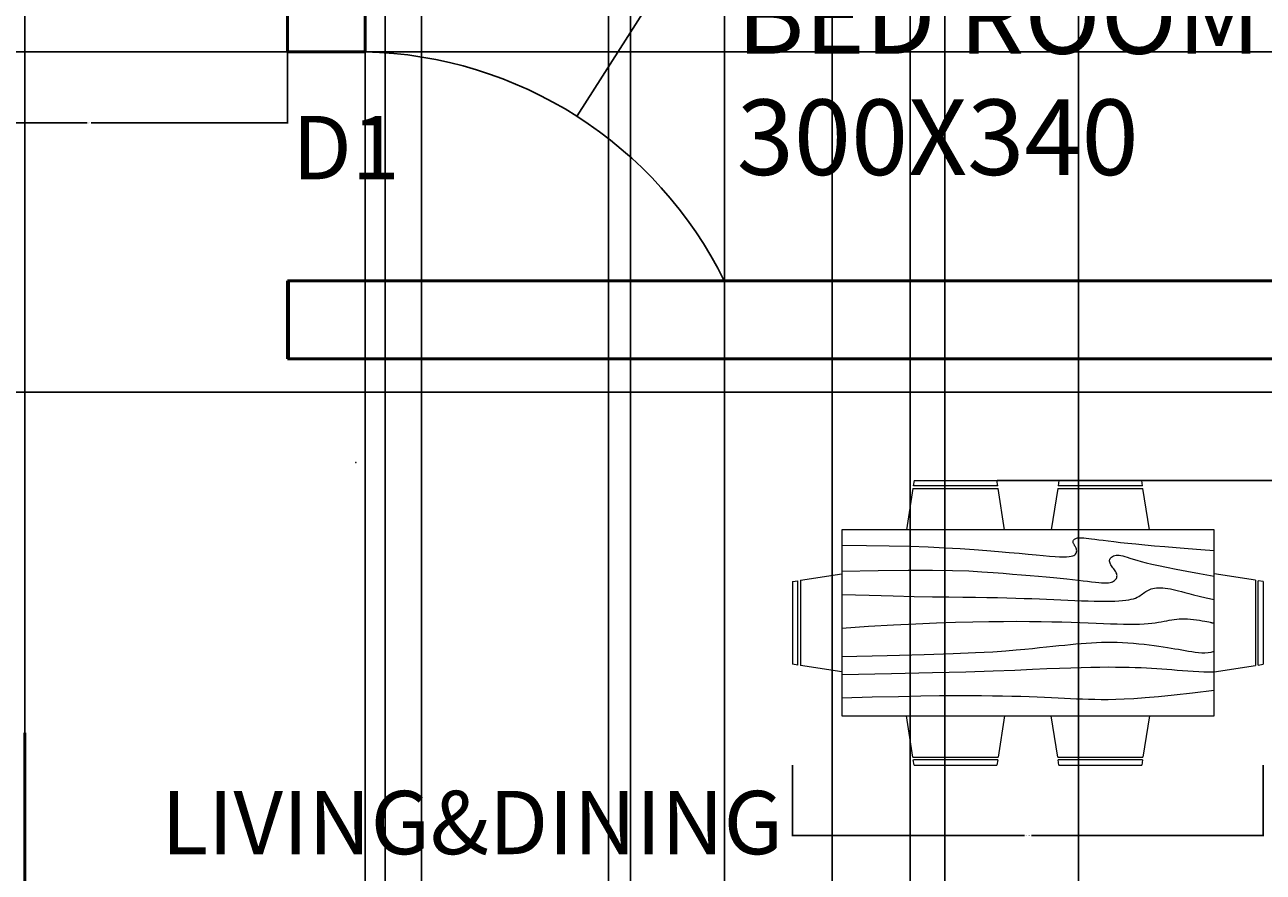
# Model space of a CAD drawing. Units: centimetres. Extents: x 2050 to 3144, y 831 to 2296.
# Tile 4 of 7: x 2553 to 2916, y 1401 to 1650. Entities that reach past the tile are written whole.
import ezdxf

# ---------------------------------------------------------------- set-up
doc = ezdxf.new("R2010")
doc.units = ezdxf.units.CM
for name, color, linetype, lineweight in [('A-ANNO-DIMS', 2, 'Continuous', 18), ('A-ANNO-TEXT', 7, 'Continuous', 18), ('A-AREA-IDEN', 7, 'Continuous', 25), ('A-DOOR', 3, 'Continuous', 25), ('A-FURN', 8, 'Continuous', 18), ('A-WALL', 7, 'Continuous', 50)]:
    doc.layers.add(name, color=color, linetype=linetype, lineweight=lineweight)
doc.styles.get("Standard").update_dxf_attribs({"font": 'arial.ttf'})
doc.dimstyles.get("Standard").update_dxf_attribs({"dimtxt": 0.18, "dimasz": 0.18, "dimexe": 0.18, "dimexo": 0.0625, "dimgap": 0.09, "dimtad": 0, "dimtih": 1, "dimtoh": 1, "dimdec": 4, "dimzin": 0, "dimdsep": 46, "dimtxsty": 'Standard', "dimcen": 0.09, "dimadec": 0, "dimazin": 0, "dimtfac": 1, "dimtdec": 4, "dimtofl": 0, "dimtmove": 0, "dimatfit": 3, "dimfxl": 1, "dimtolj": 1, "dimtzin": 0, "dimarcsym": 0})

# ---------------------------------------------------------------- blocks, each defined once
blk = doc.blocks.new('Dining Set - 36 x 72 in.')
for p, q in [((-22, 27.5), (-22.1562, 26.50042)), ((-5.8416, 26.5), (-22.1534, 26.5)), ((-22, 27.5), (-6, 27.5)), ((-5.8437, 26.49966), (-6, 27.5)), ((6, 27.5), (5.8438, 26.50042)), ((22.1584, 26.5), (5.8466, 26.5)), ((6, 27.5), (22, 27.5)), ((22.1563, 26.49966), (22, 27.5)), ((-22.2343, 26.00059), (-23.4847, 17.99762)), ((-22.2304, 26), (-5.7608, 26)), ((-4.5152, 17.99762), (-5.7655, 25.99926)), ((5.7657, 26.00059), (4.5153, 17.99762)), ((5.7696, 26), (22.2392, 26)), ((23.4848, 17.99762), (22.2345, 25.99926)), ((36, 18), (-36, 18)), ((-36, 18), (-36, -18)), ((36, -18), (36, 18)), ((-45.5, 8), (-44.5004, 8.15617)), ((-45.5, 8), (-45.5, -8)), ((-44.5, -8.15843), (-44.5, 8.15338)), ((-44.0006, 8.23428), (-35.9976, 9.48474)), ((-44, 8.23041), (-44, -8.23915)), ((44.0006, 8.23428), (35.9976, 9.48474)), ((44, 8.23041), (44, -8.23915)), ((44.5, -8.15843), (44.5, 8.15338)), ((45.5, 8), (44.5005, 8.15617)), ((45.5, 8), (45.5, -8)), ((-44.4997, -8.15631), (-45.5, -8)), ((-35.9976, -9.48476), (-43.9993, -8.2345)), ((35.9976, -9.48476), (43.9993, -8.2345)), ((44.4997, -8.15631), (45.5, -8)), ((-36, -18), (36, -18)), ((-22.2343, -26.0006), (-23.4847, -17.99762)), ((-4.5152, -17.99762), (-5.7655, -25.99928)), ((5.7657, -26.0006), (4.5153, -17.99762)), ((23.4848, -17.99762), (22.2345, -25.99928)), ((-22.2304, -26), (-5.7608, -26)), ((5.7696, -26), (22.2392, -26)), ((-22, -27.5), (-22.1562, -26.50044)), ((-5.8416, -26.5), (-22.1534, -26.5)), ((-22, -27.5), (-6, -27.5)), ((-5.8437, -26.49967), (-6, -27.5)), ((6, -27.5), (5.8438, -26.50044)), ((22.1584, -26.5), (5.8466, -26.5)), ((6, -27.5), (22, -27.5)), ((22.1563, -26.49967), (22, -27.5))]:
    blk.add_line(p, q)
for points in [[(-36, 15), (-31.1772, 14.97754), (-26.8079, 14.91406), (-22.8538, 14.81543), (-19.276, 14.6875), (-16.0362, 14.53613), (-13.0957, 14.36718), (-10.4159, 14.18652), (-7.9583, 14), (-5.6904, 13.81315), (-3.6035, 13.63021), (-1.6954, 13.45508), (0.0365, 13.29166), (1.5945, 13.14388), (2.9811, 13.01562), (4.1988, 12.9108), (5.25, 12.83333), (6.1393, 12.78613), (6.8802, 12.76823), (7.4883, 12.77767), (7.9792, 12.8125), (8.3685, 12.87077), (8.6719, 12.95052), (8.9049, 13.0498), (9.0833, 13.16666), (9.2205, 13.29899), (9.3216, 13.44401), (9.3895, 13.59879), (9.4271, 13.76041), (9.4373, 13.92594), (9.4232, 14.09245), (9.3875, 14.257), (9.3333, 14.41666), (9.2638, 14.56917), (9.1836, 14.71484), (9.0975, 14.85465), (9.0104, 14.98958), (8.9272, 15.1206), (8.8529, 15.2487), (8.7922, 15.37483), (8.75, 15.5), (8.7305, 15.62467), (8.7344, 15.74739), (8.7617, 15.86621), (8.8125, 15.97916), (8.8867, 16.08431), (8.9844, 16.17968), (9.1055, 16.26334), (9.25, 16.33333), (9.4189, 16.38802), (9.6172, 16.42708), (9.8506, 16.45052), (10.125, 16.45833), (10.4463, 16.45052), (10.8203, 16.42708), (11.2529, 16.38802), (11.75, 16.33333), (12.3184, 16.26318), (12.9694, 16.17838), (13.7151, 16.07991), (14.5677, 15.96875), (15.5395, 15.84586), (16.6426, 15.71224), (17.8893, 15.56884), (19.2917, 15.41666), (20.859, 15.25667), (22.5879, 15.08984), (24.4721, 14.91715), (26.5052, 14.73958), (28.6809, 14.5581), (30.9929, 14.3737), (33.4347, 14.18733), (36, 14)], [(-36, 10), (-28.9766, 10.14274), (-23.1725, 10.20442), (-18.4241, 10.19775), (-14.5677, 10.13541), (-11.4399, 10.03011), (-8.877, 9.89453), (-6.7154, 9.74137), (-4.7917, 9.58333), (-2.9698, 9.43082), (-1.2246, 9.28515), (0.4415, 9.14534), (2.026, 9.01041), (3.5266, 8.87939), (4.9408, 8.7513), (6.266, 8.62516), (7.5, 8.5), (8.6411, 8.37549), (9.6914, 8.2539), (10.6538, 8.13818), (11.5312, 8.03125), (12.3267, 7.93603), (13.043, 7.85547), (13.6831, 7.79248), (14.25, 7.75), (14.7471, 7.7303), (15.1797, 7.73307), (15.5537, 7.75732), (15.875, 7.80208), (16.1494, 7.86637), (16.3828, 7.94922), (16.5811, 8.04964), (16.75, 8.16666), (16.8944, 8.29915), (17.0143, 8.44531), (17.1089, 8.60319), (17.1771, 8.77083), (17.218, 8.94629), (17.2305, 9.1276), (17.2137, 9.31282), (17.1667, 9.5), (17.0895, 9.6875), (16.987, 9.875), (16.8649, 10.0625), (16.7292, 10.25), (16.5856, 10.4375), (16.4401, 10.625), (16.2985, 10.8125), (16.1667, 11), (16.05, 11.18733), (15.9518, 11.3737), (15.8752, 11.5581), (15.8229, 11.73958), (15.798, 11.91715), (15.8034, 12.08984), (15.842, 12.25667), (15.9167, 12.41666), (16.0295, 12.56836), (16.1784, 12.70833), (16.3605, 12.83268), (16.5729, 12.9375), (16.8127, 13.01888), (17.0768, 13.07291), (17.3625, 13.0957), (17.6667, 13.08333), (17.9894, 13.03312), (18.3418, 12.94726), (18.7382, 12.82918), (19.1927, 12.68229), (19.7195, 12.51001), (20.3327, 12.31575), (21.0465, 12.10294), (21.875, 11.875), (22.8357, 11.63354), (23.959, 11.37304), (25.2786, 11.08618), (26.8282, 10.76562), (28.6414, 10.40405), (30.752, 9.99414), (33.1936, 9.52856), (36, 9)], [(-36, 5.5), (-30.7157, 5.3348), (-26.069, 5.20963), (-21.9946, 5.11767), (-18.4271, 5.05208), (-15.3009, 5.00602), (-12.5508, 4.97265), (-10.1112, 4.94515), (-7.9167, 4.91666), (-5.909, 4.88167), (-4.0586, 4.83984), (-2.3429, 4.79215), (-0.7396, 4.73958), (0.7739, 4.6831), (2.22, 4.6237), (3.6213, 4.56233), (5, 4.5), (6.373, 4.43782), (7.7344, 4.3776), (9.0723, 4.32129), (10.375, 4.27083), (11.6309, 4.22819), (12.8281, 4.19531), (13.9551, 4.17415), (15, 4.16666), (15.954, 4.17448), (16.819, 4.19791), (17.6001, 4.23698), (18.3021, 4.29166), (18.9299, 4.36198), (19.4883, 4.44791), (19.9823, 4.54948), (20.4167, 4.66666), (20.7969, 4.79899), (21.1302, 4.94401), (21.4245, 5.09879), (21.6875, 5.26041), (21.9271, 5.42594), (22.1511, 5.59245), (22.3672, 5.757), (22.5834, 5.91666), (22.8065, 6.06868), (23.0404, 6.21093), (23.2879, 6.34147), (23.5521, 6.45833), (23.8358, 6.55957), (24.142, 6.64323), (24.4735, 6.70735), (24.8334, 6.75), (25.2235, 6.76969), (25.642, 6.76692), (26.0858, 6.74267), (26.5521, 6.69791), (27.0379, 6.63362), (27.5404, 6.55078), (28.0565, 6.45036), (28.5834, 6.33333), (29.1242, 6.19987), (29.7071, 6.04687), (30.3661, 5.87044), (31.1354, 5.66666), (32.0493, 5.43164), (33.142, 5.16146), (34.4475, 4.85221), (36, 4.5)], [(-36, -1), (-30.7915, -0.6591), (-26.0195, -0.38216), (-21.6519, -0.16284), (-17.6563, 0.00521), (-14.0005, 0.12833), (-10.6523, 0.21289), (-7.5796, 0.26522), (-4.75, 0.29166), (-2.134, 0.29793), (0.2878, 0.28711), (2.5317, 0.26163), (4.6146, 0.22396), (6.5529, 0.17651), (8.3633, 0.12174), (10.0623, 0.06209), (11.6667, 0), (13.1899, -0.06201), (14.6341, -0.1211), (15.9982, -0.17432), (17.2813, -0.21875), (18.4823, -0.25147), (19.6003, -0.26953), (20.6343, -0.27002), (21.5834, -0.25), (22.4481, -0.20768), (23.2357, -0.14584), (23.9549, -0.06836), (24.6146, 0.02083), (25.2235, 0.11784), (25.7904, 0.21875), (26.3241, 0.31966), (26.8334, 0.41666), (27.3265, 0.50618), (27.8099, 0.58593), (28.2894, 0.65397), (28.7709, 0.70833), (29.2601, 0.74707), (29.763, 0.76823), (30.2855, 0.76985), (30.8334, 0.75), (31.4088, 0.70784), (31.9994, 0.64713), (32.589, 0.57275), (33.1615, 0.48958), (33.7008, 0.4025), (34.1908, 0.3164), (34.6153, 0.23616), (34.9584, 0.16666), (35.2099, 0.11165), (35.3848, 0.07031), (35.504, 0.04069), (35.5886, 0.02083), (35.6594, 0.00879), (35.7377, 0.0026), (35.8442, 0.00032), (36, 0)], [(-36, -6.5), (-27.1843, -6.31267), (-20.084, -6.1263), (-14.469, -5.9419), (-10.1094, -5.76042), (-6.7752, -5.58285), (-4.2363, -5.41016), (-2.2629, -5.24333), (-0.625, -5.08334), (0.8708, -4.93099), (2.2715, -4.78646), (3.5872, -4.64974), (4.8281, -4.52084), (6.0046, -4.39974), (7.127, -4.28646), (8.2053, -4.18099), (9.25, -4.08334), (10.2705, -3.99382), (11.2734, -3.91407), (12.2647, -3.84603), (13.25, -3.79167), (14.2354, -3.75293), (15.2266, -3.73177), (16.2295, -3.73015), (17.25, -3.75), (18.2912, -3.79248), (19.3451, -3.85547), (20.4009, -3.93604), (21.4479, -4.03125), (22.4754, -4.13819), (23.4727, -4.25391), (24.4289, -4.37549), (25.3334, -4.5), (26.1785, -4.62492), (26.9694, -4.74935), (27.7145, -4.87281), (28.4219, -4.99479), (29.1, -5.11483), (29.7572, -5.23242), (30.4016, -5.34709), (31.0417, -5.45834), (31.6837, -5.56437), (32.3262, -5.65821), (32.9658, -5.73153), (33.599, -5.77604), (34.2224, -5.78345), (34.8327, -5.74545), (35.4264, -5.65373), (36, -5.5)], [(-36, -10), (-26.4022, -9.81299), (-18.4675, -9.62891), (-11.9839, -9.45069), (-6.7396, -9.28125), (-2.5226, -9.12354), (0.8789, -8.98047), (3.6769, -8.85498), (6.0833, -8.75), (8.2767, -8.66765), (10.3021, -8.60677), (12.1712, -8.56543), (13.8958, -8.54167), (15.4876, -8.53353), (16.9583, -8.53907), (18.3197, -8.55632), (19.5834, -8.58334), (20.7616, -8.61841), (21.8685, -8.66081), (22.9188, -8.71004), (23.9271, -8.76563), (24.9081, -8.82707), (25.8763, -8.89388), (26.8465, -8.96558), (27.8334, -9.04167), (28.8474, -9.12118), (29.8828, -9.20117), (30.93, -9.27824), (31.9792, -9.34896), (33.0205, -9.40991), (34.0443, -9.45768), (35.0407, -9.48885), (36, -9.5)], [(-36, -14.5), (-30.0881, -14.33513), (-25.0332, -14.21224), (-20.7312, -14.12647), (-17.0781, -14.07292), (-13.97, -14.04671), (-11.3027, -14.04297), (-8.9724, -14.05681), (-6.875, -14.08334), (-4.9224, -14.11833), (-3.0905, -14.16016), (-1.3709, -14.20785), (0.2448, -14.26042), (1.7647, -14.3169), (3.1973, -14.3763), (4.5507, -14.43767), (5.8333, -14.5), (7.0554, -14.5621), (8.235, -14.62175), (9.3922, -14.67652), (10.5469, -14.72396), (11.7192, -14.76164), (12.929, -14.78711), (14.1965, -14.79794), (15.5417, -14.79167), (16.9933, -14.76424), (18.6152, -14.70508), (20.4804, -14.60197), (22.6615, -14.44271), (25.2312, -14.21509), (28.2624, -13.9069), (31.8277, -13.50594), (36, -13)]]:
    blk.add_lwpolyline(points)
blk = doc.blocks.new('DOOR-D1-1165')
blk.add_line((116.51, 0), (116.51, 139.37))
blk.add_arc((116.51, 116.51), 116.51, 180, 270)
blk = doc.blocks.new('*D16')
at = {"layer": 'A-ANNO-DIMS', "color": 0, "lineweight": -2, "transparency": 16777216}
for p, q in [((2513.36, 1641.97), (2513.36, 1620.95)), ((2629.87, 1641.97), (2629.87, 1620.95)), ((2513.54, 1621.13), (2571.02, 1621.13)), ((2629.69, 1621.13), (2572.2, 1621.13))]:
    blk.add_line(p, q, dxfattribs=at)
at = {"layer": 'A-ANNO-DIMS', "color": 0, "transparency": 16777216}
for points in [[(2513.54, 1621.16), (2513.54, 1621.1), (2513.36, 1621.13)], [(2629.69, 1621.16), (2629.69, 1621.1), (2629.87, 1621.13)]]:
    blk.add_solid(points, dxfattribs=at)
at = {"layer": 'Defpoints', "color": 0, "transparency": 16777216}
for p in [(2513.36, 1642.03), (2629.87, 1642.03), (2629.87, 1621.13)]:
    blk.add_point(p, dxfattribs=at)
at = {"layer": 'A-ANNO-DIMS', "color": 0, "transparency": 16777216, "insert": (2571.61, 1621.13), "char_height": 0.18, "attachment_point": 5}
blk.add_mtext('\\A1;117 TYP.', dxfattribs=at)
blk = doc.blocks.new('*D19')
at = {"layer": 'A-ANNO-DIMS', "color": 0, "lineweight": -2, "transparency": 16777216}
for p, q in [((2778.22, 1432.48), (2778.22, 1411.63)), ((2916.44, 1432.48), (2916.44, 1411.63)), ((2778.4, 1411.81), (2846.29, 1411.81)), ((2916.26, 1411.81), (2848.37, 1411.81))]:
    blk.add_line(p, q, dxfattribs=at)
at = {"layer": 'A-ANNO-DIMS', "color": 0, "transparency": 16777216}
for points in [[(2778.4, 1411.84), (2778.4, 1411.78), (2778.22, 1411.81)], [(2916.26, 1411.84), (2916.26, 1411.78), (2916.44, 1411.81)]]:
    blk.add_solid(points, dxfattribs=at)
at = {"layer": 'Defpoints', "color": 0, "transparency": 16777216}
for p in [(2778.22, 1432.54), (2916.44, 1432.54), (2916.44, 1411.81)]:
    blk.add_point(p, dxfattribs=at)
at = {"layer": 'A-ANNO-DIMS', "color": 0, "transparency": 16777216, "insert": (2847.33, 1411.81), "char_height": 0.18, "attachment_point": 5}
blk.add_mtext('\\A1;DINING SET 138', dxfattribs=at)
blk = doc.blocks.new('*D48')
at = {"layer": 'A-ANNO-DIMS', "color": 0, "lineweight": -2, "transparency": 16777216}
for p, q in [((2552.73, 1211.94), (2552.73, 2154.53)), ((2552.91, 2154.35), (2610.59, 2154.35)), ((2669.05, 2154.35), (2611.37, 2154.35)), ((2669.23, 1211.94), (2669.23, 2154.53))]:
    blk.add_line(p, q, dxfattribs=at)
at = {"layer": 'A-ANNO-DIMS', "color": 0, "transparency": 16777216}
for points in [[(2552.91, 2154.38), (2552.91, 2154.32), (2552.73, 2154.35)], [(2669.05, 2154.38), (2669.05, 2154.32), (2669.23, 2154.35)]]:
    blk.add_solid(points, dxfattribs=at)
at = {"layer": 'Defpoints', "color": 0, "transparency": 16777216}
for p in [(2669.23, 2154.35), (2552.73, 1211.87), (2669.23, 1211.87)]:
    blk.add_point(p, dxfattribs=at)
at = {"layer": 'A-ANNO-DIMS', "color": 0, "transparency": 16777216, "insert": (2610.98, 2154.35), "char_height": 0.18, "attachment_point": 5}
blk.add_mtext('\\A1;116.5', dxfattribs=at)
blk = doc.blocks.new('*D52')
at = {"layer": 'A-ANNO-DIMS', "color": 0, "lineweight": -2, "transparency": 16777216}
for p, q in [((2513.42, 1642.03), (3042.37, 1642.03)), ((3042.19, 1641.85), (3042.19, 1592.22)), ((3042.19, 1542.21), (3042.19, 1591.85)), ((2513.42, 1542.03), (3042.37, 1542.03))]:
    blk.add_line(p, q, dxfattribs=at)
at = {"layer": 'A-ANNO-DIMS', "color": 0, "transparency": 16777216}
for points in [[(3042.16, 1641.85), (3042.22, 1641.85), (3042.19, 1642.03)], [(3042.16, 1542.21), (3042.22, 1542.21), (3042.19, 1542.03)]]:
    blk.add_solid(points, dxfattribs=at)
at = {"layer": 'Defpoints', "color": 0, "transparency": 16777216}
for p in [(2513.36, 1642.03), (3042.19, 1642.03), (2513.36, 1542.03)]:
    blk.add_point(p, dxfattribs=at)
at = {"layer": 'A-ANNO-DIMS', "color": 0, "transparency": 16777216, "insert": (3042.19, 1592.03), "char_height": 0.18, "attachment_point": 5}
blk.add_mtext('\\A1;100', dxfattribs=at)
blk = doc.blocks.new('*D56')
at = {"layer": 'A-ANNO-DIMS', "color": 0, "lineweight": -2, "transparency": 16777216}
for p, q in [((2652.79, 1642.03), (3042.37, 1642.03)), ((3042.19, 1641.85), (3042.19, 1608.57)), ((3042.19, 1574.91), (3042.19, 1608.2)), ((2630.24, 1574.73), (3042.37, 1574.73))]:
    blk.add_line(p, q, dxfattribs=at)
at = {"layer": 'A-ANNO-DIMS', "color": 0, "transparency": 16777216}
for points in [[(3042.16, 1641.85), (3042.22, 1641.85), (3042.19, 1642.03)], [(3042.16, 1574.91), (3042.22, 1574.91), (3042.19, 1574.73)]]:
    blk.add_solid(points, dxfattribs=at)
at = {"layer": 'Defpoints', "color": 0, "transparency": 16777216}
for p in [(2652.73, 1642.03), (2630.18, 1574.73), (3042.19, 1574.73)]:
    blk.add_point(p, dxfattribs=at)
at = {"layer": 'A-ANNO-DIMS', "color": 0, "transparency": 16777216, "insert": (3042.19, 1608.38), "char_height": 0.18, "attachment_point": 5}
blk.add_mtext('\\A1;67.3', dxfattribs=at)
blk = doc.blocks.new('*D58')
at = {"layer": 'A-ANNO-DIMS', "color": 0, "lineweight": -2, "transparency": 16777216}
for p, q in [((2952.79, 1551.87), (3042.37, 1551.87)), ((3042.19, 1551.69), (3042.19, 1534.16)), ((3042.19, 1516.26), (3042.19, 1533.8)), ((2838.28, 1516.08), (3042.37, 1516.08))]:
    blk.add_line(p, q, dxfattribs=at)
at = {"layer": 'A-ANNO-DIMS', "color": 0, "transparency": 16777216}
for points in [[(3042.16, 1551.69), (3042.22, 1551.69), (3042.19, 1551.87)], [(3042.16, 1516.26), (3042.22, 1516.26), (3042.19, 1516.08)]]:
    blk.add_solid(points, dxfattribs=at)
at = {"layer": 'Defpoints', "color": 0, "transparency": 16777216}
for p in [(2952.73, 1551.87), (3042.19, 1551.87), (2838.22, 1516.08)]:
    blk.add_point(p, dxfattribs=at)
at = {"layer": 'A-ANNO-DIMS', "color": 0, "transparency": 16777216, "insert": (3042.19, 1533.98), "char_height": 0.18, "attachment_point": 5}
blk.add_mtext('\\A1;35.794', dxfattribs=at)
blk = doc.blocks.new('*D59')
at = {"layer": 'A-ANNO-DIMS', "color": 0, "lineweight": -2, "transparency": 16777216}
for p, q in [((2862.15, 1253.11), (2862.15, 2154.53)), ((2862.33, 2154.35), (2907.04, 2154.35)), ((2952.55, 2154.35), (2907.83, 2154.35)), ((2952.73, 1211.94), (2952.73, 2154.53))]:
    blk.add_line(p, q, dxfattribs=at)
at = {"layer": 'A-ANNO-DIMS', "color": 0, "transparency": 16777216}
for points in [[(2862.33, 2154.38), (2862.33, 2154.32), (2862.15, 2154.35)], [(2952.55, 2154.38), (2952.55, 2154.32), (2952.73, 2154.35)]]:
    blk.add_solid(points, dxfattribs=at)
at = {"layer": 'Defpoints', "color": 0, "transparency": 16777216}
for p in [(2952.73, 2154.35), (2862.15, 1253.05), (2952.73, 1211.87)]:
    blk.add_point(p, dxfattribs=at)
at = {"layer": 'A-ANNO-DIMS', "color": 0, "transparency": 16777216, "insert": (2907.44, 2154.35), "char_height": 0.18, "attachment_point": 5}
blk.add_mtext('\\A1;90.58', dxfattribs=at)
blk = doc.blocks.new('*D61')
at = {"layer": 'A-ANNO-DIMS', "color": 0, "lineweight": -2, "transparency": 16777216}
for p, q in [((2552.73, 1328.44), (2552.73, 2154.53)), ((2552.91, 2154.35), (2638.04, 2154.35)), ((2723.95, 2154.35), (2638.81, 2154.35)), ((2724.13, 1334.5), (2724.13, 2154.53))]:
    blk.add_line(p, q, dxfattribs=at)
at = {"layer": 'A-ANNO-DIMS', "color": 0, "transparency": 16777216}
for points in [[(2552.91, 2154.38), (2552.91, 2154.32), (2552.73, 2154.35)], [(2723.95, 2154.38), (2723.95, 2154.32), (2724.13, 2154.35)]]:
    blk.add_solid(points, dxfattribs=at)
at = {"layer": 'Defpoints', "color": 0, "transparency": 16777216}
for p in [(2724.13, 2154.35), (2724.13, 1334.43), (2552.73, 1328.38)]:
    blk.add_point(p, dxfattribs=at)
at = {"layer": 'A-ANNO-DIMS', "color": 0, "transparency": 16777216, "insert": (2638.43, 2154.35), "char_height": 0.18, "attachment_point": 5}
blk.add_mtext('\\A1;171.4', dxfattribs=at)
blk = doc.blocks.new('*D62')
at = {"layer": 'A-ANNO-DIMS', "color": 0, "lineweight": -2, "transparency": 16777216}
for p, q in [((2758.2, 1334.5), (2758.2, 2154.53)), ((2758.38, 2154.35), (2773.58, 2154.35)), ((2789.71, 2154.35), (2774.51, 2154.35)), ((2789.89, 1319.12), (2789.89, 2154.53))]:
    blk.add_line(p, q, dxfattribs=at)
at = {"layer": 'A-ANNO-DIMS', "color": 0, "transparency": 16777216}
for points in [[(2758.38, 2154.38), (2758.38, 2154.32), (2758.2, 2154.35)], [(2789.71, 2154.38), (2789.71, 2154.32), (2789.89, 2154.35)]]:
    blk.add_solid(points, dxfattribs=at)
at = {"layer": 'Defpoints', "color": 0, "transparency": 16777216}
for p in [(2789.89, 2154.35), (2758.2, 1334.43), (2789.89, 1319.06)]:
    blk.add_point(p, dxfattribs=at)
at = {"layer": 'A-ANNO-DIMS', "color": 0, "transparency": 16777216, "insert": (2774.05, 2154.35), "char_height": 0.18, "attachment_point": 5}
blk.add_mtext('\\A1;31.696', dxfattribs=at)
blk = doc.blocks.new('*D65')
at = {"layer": 'A-ANNO-DIMS', "color": 0, "lineweight": -2, "transparency": 16777216}
for p, q in [((2812.73, 1924.83), (2812.73, 1009.53)), ((2822.89, 1914.67), (2822.89, 1009.53)), ((2812.91, 1009.71), (2817.42, 1009.71)), ((2822.71, 1009.71), (2818.19, 1009.71))]:
    blk.add_line(p, q, dxfattribs=at)
at = {"layer": 'A-ANNO-DIMS', "color": 0, "transparency": 16777216}
for points in [[(2812.91, 1009.74), (2812.91, 1009.68), (2812.73, 1009.71)], [(2822.71, 1009.74), (2822.71, 1009.68), (2822.89, 1009.71)]]:
    blk.add_solid(points, dxfattribs=at)
at = {"layer": 'Defpoints', "color": 0, "transparency": 16777216}
for p in [(2812.73, 1924.89), (2822.89, 1914.73), (2822.89, 1009.71)]:
    blk.add_point(p, dxfattribs=at)
at = {"layer": 'A-ANNO-DIMS', "color": 0, "transparency": 16777216, "insert": (2817.81, 1009.71), "char_height": 0.18, "attachment_point": 5}
blk.add_mtext('\\A1;10.16', dxfattribs=at)
blk = doc.blocks.new('*D68')
at = {"layer": 'A-ANNO-DIMS', "color": 0, "lineweight": -2, "transparency": 16777216}
for p, q in [((2652.73, 1914.67), (2652.73, 1009.53)), ((2730.58, 1841.3), (2730.58, 1009.53)), ((2652.91, 1009.71), (2691.26, 1009.71)), ((2730.4, 1009.71), (2692.05, 1009.71))]:
    blk.add_line(p, q, dxfattribs=at)
at = {"layer": 'A-ANNO-DIMS', "color": 0, "transparency": 16777216}
for points in [[(2652.91, 1009.74), (2652.91, 1009.68), (2652.73, 1009.71)], [(2730.4, 1009.74), (2730.4, 1009.68), (2730.58, 1009.71)]]:
    blk.add_solid(points, dxfattribs=at)
at = {"layer": 'Defpoints', "color": 0, "transparency": 16777216}
for p in [(2652.73, 1914.73), (2730.58, 1841.36), (2730.58, 1009.71)]:
    blk.add_point(p, dxfattribs=at)
at = {"layer": 'A-ANNO-DIMS', "color": 0, "transparency": 16777216, "insert": (2691.65, 1009.71), "char_height": 0.18, "attachment_point": 5}
blk.add_mtext('\\A1;77.85', dxfattribs=at)
blk = doc.blocks.new('*D73')
at = {"layer": 'A-ANNO-DIMS', "color": 0, "lineweight": -2, "transparency": 16777216}
for p, q in [((2658.57, 1971.45), (2658.57, 1009.53)), ((2652.73, 1924.83), (2652.73, 1009.53)), ((2652.91, 1009.71), (2655.26, 1009.71)), ((2658.39, 1009.71), (2656.04, 1009.71))]:
    blk.add_line(p, q, dxfattribs=at)
at = {"layer": 'A-ANNO-DIMS', "color": 0, "transparency": 16777216}
for points in [[(2652.91, 1009.74), (2652.91, 1009.68), (2652.73, 1009.71)], [(2658.39, 1009.74), (2658.39, 1009.68), (2658.57, 1009.71)]]:
    blk.add_solid(points, dxfattribs=at)
at = {"layer": 'Defpoints', "color": 0, "transparency": 16777216}
for p in [(2658.57, 1971.51), (2652.73, 1924.89), (2658.57, 1009.71)]:
    blk.add_point(p, dxfattribs=at)
at = {"layer": 'A-ANNO-DIMS', "color": 0, "transparency": 16777216, "insert": (2655.65, 1009.71), "char_height": 0.18, "attachment_point": 5}
blk.add_mtext('\\A1;5.847', dxfattribs=at)
blk = doc.blocks.new('*D74')
at = {"layer": 'A-ANNO-DIMS', "color": 0, "lineweight": -2, "transparency": 16777216}
for p, q in [((2952.73, 2064.83), (2952.73, 1009.53)), ((2822.89, 2004.16), (2822.89, 1009.53)), ((2823.07, 1009.71), (2887.35, 1009.71)), ((2952.55, 1009.71), (2888.26, 1009.71))]:
    blk.add_line(p, q, dxfattribs=at)
at = {"layer": 'A-ANNO-DIMS', "color": 0, "transparency": 16777216}
for points in [[(2823.07, 1009.74), (2823.07, 1009.68), (2822.89, 1009.71)], [(2952.55, 1009.74), (2952.55, 1009.68), (2952.73, 1009.71)]]:
    blk.add_solid(points, dxfattribs=at)
at = {"layer": 'Defpoints', "color": 0, "transparency": 16777216}
for p in [(2952.73, 2064.89), (2822.89, 2004.22), (2952.73, 1009.71)]:
    blk.add_point(p, dxfattribs=at)
at = {"layer": 'A-ANNO-DIMS', "color": 0, "transparency": 16777216, "insert": (2887.81, 1009.71), "char_height": 0.18, "attachment_point": 5}
blk.add_mtext('\\A1;129.84', dxfattribs=at)
blk = doc.blocks.new('*D76')
at = {"layer": 'A-ANNO-DIMS', "color": 0, "lineweight": -2, "transparency": 16777216}
for p, q in [((2753.78, 1684.12), (2714.94, 1623.27)), ((2753.96, 1684.12), (2753.78, 1684.12)), ((2649.86, 1521.45), (2650.04, 1521.45)), ((2649.95, 1521.36), (2649.95, 1521.54))]:
    blk.add_line(p, q, dxfattribs=at)
at = {"layer": 'A-ANNO-DIMS', "color": 0, "transparency": 16777216}
blk.add_solid([(2714.92, 1623.29), (2714.97, 1623.25), (2714.85, 1623.12)], dxfattribs=at)
at = {"layer": 'Defpoints', "color": 0, "transparency": 16777216}
for p in [(2714.85, 1623.12), (2649.95, 1521.45)]:
    blk.add_point(p, dxfattribs=at)
at = {"layer": 'A-ANNO-DIMS', "color": 0, "transparency": 16777216, "insert": (2754.5, 1684.12), "char_height": 0.18, "attachment_point": 5}
blk.add_mtext('\\A1;R120.61', dxfattribs=at)

msp = doc.modelspace()

# ---------------------------------------------------------------- linework, layer by layer
at = {"layer": 'A-DOOR'}
msp.add_arc((2649.9472, 1521.4533), 120.6135, 26.215835, 88.679609, dxfattribs=at)
at = {"layer": 'A-WALL'}
for p, q in [((2629.8665, 2064.8948), (2629.8665, 1642.0348)), ((2652.7265, 1914.7348), (2652.7265, 1642.0348)), ((2652.7265, 1642.0348), (2629.8665, 1642.0348)), ((2952.7265, 1574.7348), (2629.8665, 1574.7348)), ((2629.8665, 1574.7348), (2629.8665, 1551.8748)), ((2630.1795, 1574.7348), (2630.1795, 1551.8748)), ((2952.7265, 1551.8748), (2629.8665, 1551.8748)), ((2552.7265, 1076.3148), (2552.7265, 1442.0348))]:
    msp.add_line(p, q, dxfattribs=at)

# ---------------------------------------------------------------- block references
at = {"layer": 'A-DOOR', "extrusion": (0, 0, -1), "zscale": -1, "rotation": 180}
msp.add_blockref('DOOR-D1-1165', (-2513.361, 1781.4006), dxfattribs=at)
at = {"layer": 'A-FURN', "xscale": 1.518878716440213, "yscale": 1.518878716440213, "zscale": 1.518878716440213}
msp.add_blockref('Dining Set - 36 x 72 in.', (2847.3285, 1474.3117), dxfattribs=at)

# ---------------------------------------------------------------- texts
at = {"layer": 'A-ANNO-TEXT'}
msp.add_text('D1', height=18.59595, dxfattribs=at).set_placement((2631.2959, 1604.5892))
at = {"layer": 'A-AREA-IDEN'}
for s, height, p in [('BED ROOM', 22.16939, (2761.802, 1641.4722)), ('300X340', 22.16939, (2761.802, 1605.8591)), ('LIVING&DINING', 18.579384, (2592.7975, 1406.3703))]:
    msp.add_text(s, height=height, dxfattribs=at).set_placement(p)

# ---------------------------------------------------------------- dimensions: what is measured, and where the dimension line sits
at = {"layer": 'A-ANNO-DIMS'}
for base, p1, p2, override, picture, middle in [((2669.2319, 2154.3548), (2552.7265, 1211.8748), (2669.2319, 1211.8748), {"dimdec": 1, "dimlfac": 1, "dimrnd": 0, "dimzin": 0, "dimdsep": 46, "dimlunit": 2}, '*D48', (2610.9792, 2154.3548)), ((2724.1318, 2154.3548), (2552.7265, 1328.3801), (2724.1318, 1334.433), {"dimdec": 1, "dimlfac": 1, "dimrnd": 0, "dimzin": 0, "dimdsep": 46, "dimlunit": 2}, '*D61', (2638.4292, 2154.3548)), ((2789.8945, 2154.3548), (2758.1988, 1334.433), (2789.8945, 1319.0567), {"dimdec": 3, "dimlfac": 1, "dimrnd": 0, "dimzin": 0, "dimdsep": 46, "dimlunit": 2}, '*D62', (2774.0467, 2154.3548)), ((2952.7265, 2154.3548), (2862.1454, 1253.0515), (2952.7265, 1211.8748), {"dimdec": 2, "dimlfac": 1, "dimrnd": 0, "dimzin": 0, "dimdsep": 46, "dimlunit": 2}, '*D59', (2907.436, 2154.3548)), ((2952.7265, 1009.7148), (2822.8865, 2004.2202), (2952.7265, 2064.8948), {"dimdec": 2, "dimlfac": 1, "dimrnd": 0, "dimzin": 0, "dimdsep": 46, "dimlunit": 2}, '*D74', (2887.8065, 1009.7148)), ((2658.5737, 1009.7148), (2652.7265, 1924.8948), (2658.5737, 1971.5118), {"dimdec": 3, "dimlfac": 1, "dimrnd": 0, "dimzin": 0, "dimdsep": 46, "dimlunit": 2}, '*D73', (2655.6501, 1009.7148)), ((2822.8865, 1009.7148), (2812.7265, 1924.8948), (2822.8865, 1914.7348), {"dimdec": 2, "dimlfac": 1, "dimrnd": 0, "dimzin": 0, "dimdsep": 46, "dimlunit": 2}, '*D65', (2817.8065, 1009.7148)), ((2730.579, 1009.7148), (2652.7265, 1914.7348), (2730.579, 1841.3577), {"dimdec": 2, "dimlfac": 1, "dimrnd": 0, "dimzin": 0, "dimdsep": 46, "dimlunit": 2}, '*D68', (2691.6528, 1009.7148))]:
    dim = msp.add_linear_dim(base=base, p1=p1, p2=p2, dimstyle='Standard', override=override, dxfattribs=at)
    dim.commit()
    dim.dimension.update_dxf_attribs({"geometry": picture, "text_midpoint": middle})
dim = msp.add_radius_dim(center=(2649.9472, 1521.4533), mpoint=(2714.8457, 1623.1185), dimstyle='Standard', override={"dimdec": 2, "dimlfac": 1, "dimrnd": 0, "dimzin": 0, "dimdsep": 46, "dimlunit": 2}, dxfattribs=at)
dim.commit()
dim.dimension.update_dxf_attribs({"geometry": '*D76', "text_midpoint": (2754.4971, 1684.1176), "dimtype": 164})
for base, p1, p2, text, picture, middle in [((2629.8665, 1621.13), (2513.3612, 1642.0348), (2629.8665, 1642.0348), '<> TYP.', '*D16', (2571.6139, 1621.13)), ((2916.4375, 1411.8098), (2778.2196, 1432.5425), (2916.4375, 1432.5425), 'DINING SET <>', '*D19', (2847.3285, 1411.8098))]:
    dim = msp.add_linear_dim(base=base, p1=p1, p2=p2, text=text, dimstyle='Standard', override={"dimdec": 0, "dimlfac": 1, "dimrnd": 0, "dimzin": 0, "dimdsep": 46, "dimlunit": 2}, dxfattribs=at)
    dim.commit()
    dim.dimension.update_dxf_attribs({"geometry": picture, "text_midpoint": middle})
for base, p1, p2, override, picture, middle in [((3042.1865, 1642.0348), (2513.3612, 1542.0348), (2513.3612, 1642.0348), {"dimdec": 0, "dimlfac": 1, "dimrnd": 0, "dimzin": 0, "dimdsep": 46, "dimlunit": 2}, '*D52', (3042.1865, 1592.0348)), ((3042.1865, 1574.7348), (2652.7265, 1642.0348), (2630.1795, 1574.7348), {"dimdec": 1, "dimlfac": 1, "dimrnd": 0, "dimzin": 0, "dimdsep": 46, "dimlunit": 2}, '*D56', (3042.1865, 1608.3848)), ((3042.1865, 1551.8748), (2838.2153, 1516.0808), (2952.7265, 1551.8748), {"dimdec": 3, "dimlfac": 1, "dimrnd": 0, "dimzin": 0, "dimdsep": 46, "dimlunit": 2}, '*D58', (3042.1865, 1533.9778))]:
    dim = msp.add_linear_dim(base=base, p1=p1, p2=p2, angle=90, dimstyle='Standard', override=override, dxfattribs=at)
    dim.commit()
    dim.dimension.update_dxf_attribs({"geometry": picture, "text_midpoint": middle})

doc.saveas('drawing.dxf')
